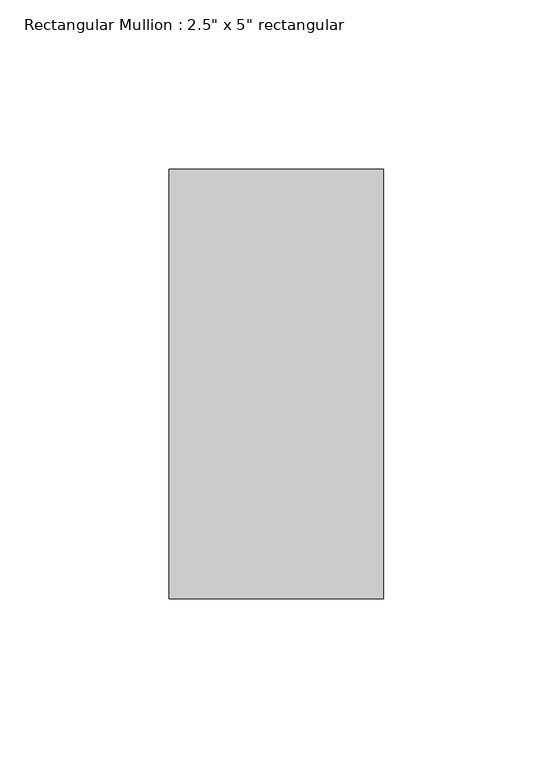
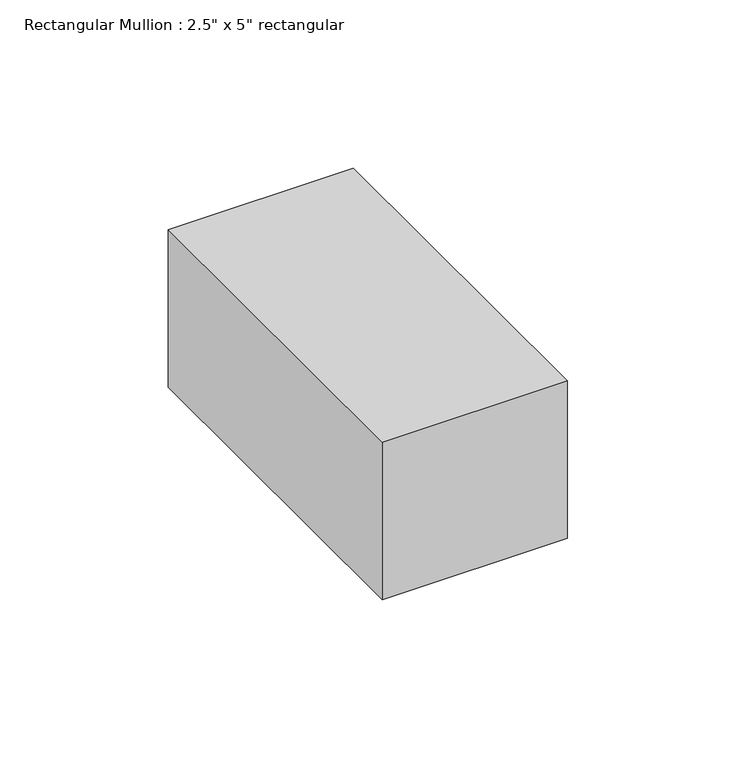
"""IFC4 building model written with IfcOpenShell, lengths in millimetres: member geometry."""

from ifc_helpers import new_model, si_unit, frame, origin, place, context, project, spatial, polyline, outline, extrude, source, transform, mapped, element, save


def member_35f02b64(model_context):
    return source(origin(), model_context, "Body", "SweptSolid", [
        extrude(outline(polyline([(0.0, 63.5), (0.0, -63.5), (-63.5, -63.5), (-63.5, 63.5), (0.0, 63.5)])), frame((0.0, 0.0, -57.15), z_axis=(0.0, 0.0, 1.0), x_axis=(1.0, 0.0, 0.0)), (0.0, 0.0, 1.0), 57.15),
    ])


if __name__ == "__main__":
    model = new_model("IFC4")
    model_context = context("Model", 3, world=origin())
    ifc_project = project(units=[si_unit("LENGTHUNIT", "METRE", prefix="MILLI")], contexts=[model_context])
    site = spatial("IfcSite", under=ifc_project)
    building = spatial("IfcBuilding", under=site)
    placement = place(None, origin())
    member_shape = member_35f02b64(model_context)
    element("IfcMember", 1, ObjectType="Rectangular Mullion : 2.5\" x 5\" rectangular", at=placement, inside=building, context=model_context, shape_type="MappedRepresentation", body=[
        mapped(member_shape, transform((0.0, 0.0, 0.0), x_axis=(1.0, 0.0, 0.0), y_axis=(0.0, 1.0, 0.0), z_axis=(0.0, 0.0, 1.0))),
    ])
    save(model, "model.ifc")

# Revit data of these elements
# Type "Rectangular Mullion : 2.5\" x 5\" rectangular"
#   built-in parameter 1007304 = 0.416667 (stored number, unit not read)
#   built-in parameter 1007301 = 0.104167 (stored number, unit not read)
#   built-in parameter 1007300 = 0.104167 (stored number, unit not read)
# Element 1 (IfcMember, "Rectangular Mullion : 2.5\" x 5\" rectangular")
#   Materials on its faces: "Aluminum"
# Materials
#   "Aluminum": class "Metal", colour RGB 247 247 247, transparency 0, Description = "Aluminum 6061", Cost = 0
